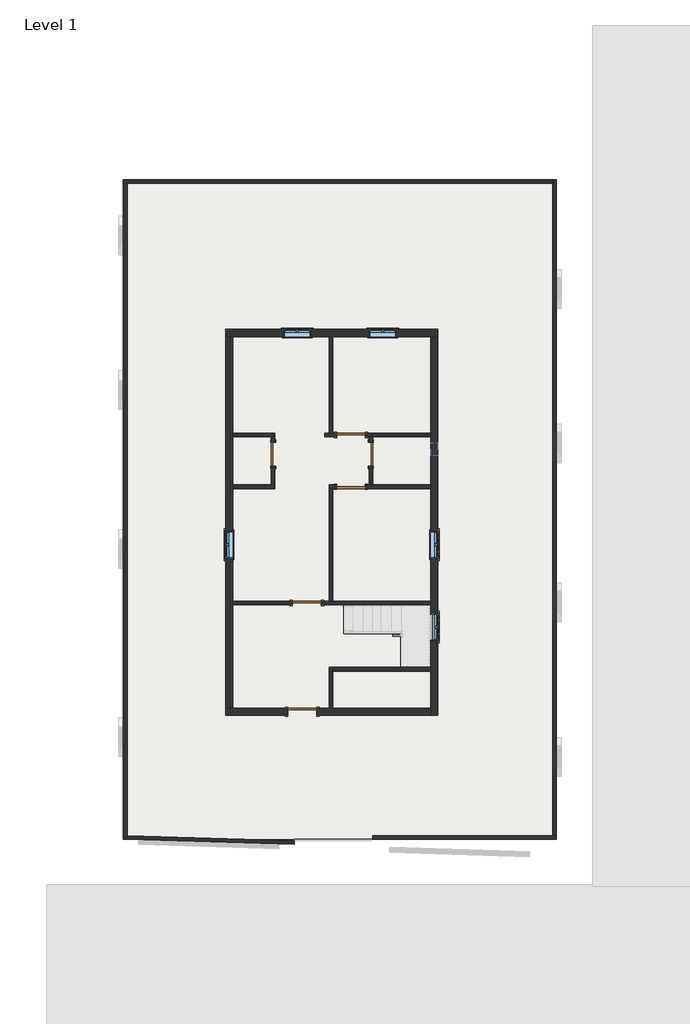
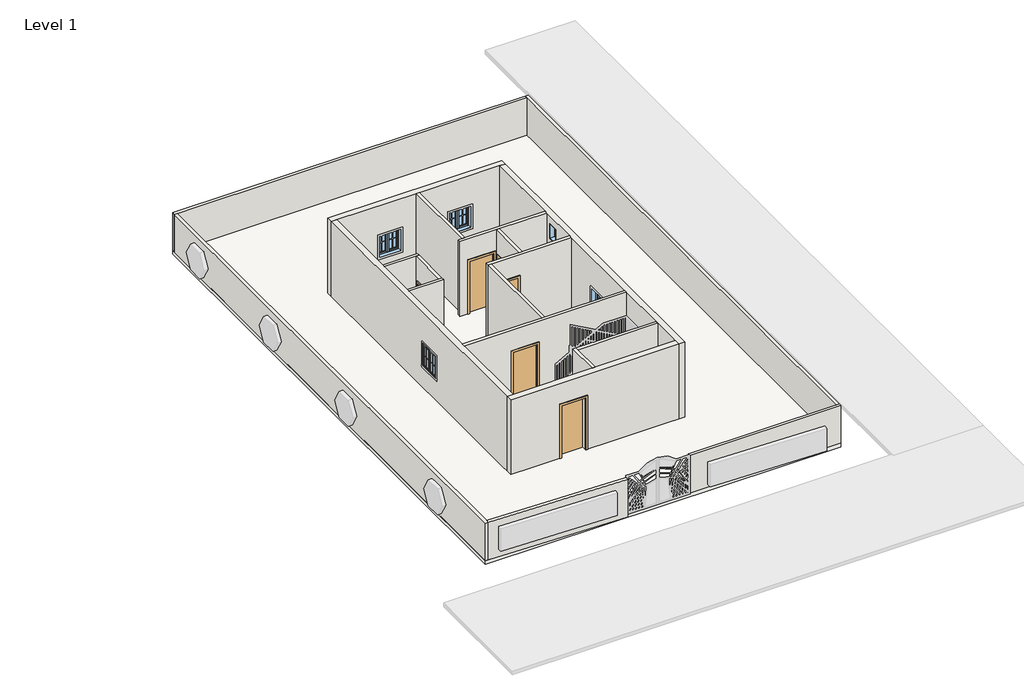
# One storey, part 1 of 3: 20 walls, 6 doors, 6 windows, 1 slab.
"""IFC4 building model written with IfcOpenShell, lengths in millimetres."""

from ifc_helpers import new_model, si_unit, frame, origin, origin_with_axes, place, context, project, spatial, polyline, outline, extrude, faceted_brep, transform, mapped, element, save
from components import door_f2b275c1, door_d8f5dbb5, door_305aa2a5, door_e5f9f3c4, door_a90ba1ad, window_aa618e30, window_339605e1

model = new_model("IFC4")

# Units and contexts
model_context = context("Model", 3, world=origin())
ifc_project = project(units=[si_unit("LENGTHUNIT", "METRE", prefix="MILLI")], contexts=[model_context])

# Site, building, storey
site = spatial("IfcSite", under=ifc_project)
building = spatial("IfcBuilding", under=site)
storey = spatial("IfcBuildingStorey", under=building, Name="Level 1", Elevation=0.0)

# Doors
placement = place(None, origin())
door_shape = door_f2b275c1(model_context)
element("IfcDoor", 1, ObjectType="Single-Flush : 30\" x 80\"", at=placement, inside=storey, context=model_context, shape_type="MappedRepresentation", body=[
    mapped(door_shape, transform((-22.290747, 2690.8435985, 0.0), x_axis=(0.0, 1.0, 0.0), y_axis=(-1.0, 0.0, 0.0), z_axis=(0.0, 0.0, 1.0))),
])
door_2_shape = door_d8f5dbb5(model_context)
element("IfcDoor", 2, ObjectType="Single-Flush : 30\" x 80\"", at=placement, inside=storey, context=model_context, shape_type="MappedRepresentation", body=[
    mapped(door_2_shape, transform((-3108.390747, 2690.8435985, 0.0), x_axis=(0.0, 1.0, 0.0), y_axis=(-1.0, 0.0, 0.0), z_axis=(0.0, 0.0, 1.0))),
])
door_3_shape = door_305aa2a5(model_context)
element("IfcDoor", 3, ObjectType="Single-Flush : 36\" x 84\"", at=placement, inside=storey, context=model_context, shape_type="MappedRepresentation", body=[
    mapped(door_3_shape, transform((-650.940747, 3300.4435985, 0.0), x_axis=(-1.0, 0.0, 0.0), y_axis=(0.0, -1.0, 0.0), z_axis=(0.0, 0.0, 1.0))),
])
door_4_shape = door_e5f9f3c4(model_context)
element("IfcDoor", 4, ObjectType="Single-Flush : 36\" x 84\"", at=placement, inside=storey, context=model_context, shape_type="MappedRepresentation", body=[
    mapped(door_4_shape, transform((-2041.590747, -2008.1564015, 0.0), x_axis=(1.0, 0.0, 0.0), y_axis=(0.0, 1.0, 0.0), z_axis=(0.0, 0.0, 1.0))),
])
element("IfcDoor", 5, ObjectType="Single-Flush : 36\" x 84\"", at=placement, inside=storey, context=model_context, shape_type="MappedRepresentation", body=[
    mapped(door_4_shape, transform((-650.940747, 1662.1435985, 0.0), x_axis=(-1.0, 0.0, 0.0), y_axis=(0.0, -1.0, 0.0), z_axis=(0.0, 0.0, 1.0))),
])
door_5_shape = door_a90ba1ad(model_context)
element("IfcDoor", 6, ObjectType="Single-Flush : 36\" x 84\"", at=placement, inside=storey, context=model_context, shape_type="MappedRepresentation", body=[
    mapped(door_5_shape, transform((-2193.990747, -5443.5064015, 0.0), x_axis=(-1.0, 0.0, 0.0), y_axis=(0.0, -1.0, 0.0), z_axis=(0.0, 0.0, 1.0))),
])

# Slab
element("IfcSlab", 7, ObjectType="Generic - 12\"", at=placement, inside=storey, context=model_context, shape_type="SweptSolid", body=[
    extrude(outline(polyline([(5837.7486397, 11368.6225468), (5837.7486397, -9472.0774532), (-7840.1513603, -9472.0774532), (-7840.1513603, 11368.6225468), (5837.7486397, 11368.6225468)])), frame((0.0, 0.0, -152.4), z_axis=(0.0, 0.0, 1.0), x_axis=(1.0, 0.0, 0.0)), (0.0, 0.0, 1.0), 152.4),
])

# Walls
element("IfcWall", 8, ObjectType="WALL4.5\"", at=placement, inside=storey, context=model_context, shape_type="Brep", body=[
    faceted_brep([(-4384.740747, 3243.2935985, 0.0), (-3165.540747, 3243.2935985, 0.0), (-3051.240747, 3243.2935985, 0.0), (-3051.240747, 3243.2935985, 3048.0), (-3165.540747, 3243.2935985, 3048.0), (-4384.740747, 3243.2935985, 3048.0), (-4384.740747, 3357.5935985, 0.0), (-4384.740747, 3357.5935985, 3048.0), (-3051.240747, 3357.5935985, 3048.0), (-3051.240747, 3357.5935985, 0.0)], [[[0, 1, 2, 3, 4, 5]], [[6, 7, 8, 9]], [[2, 1, 0, 6, 9]], [[0, 5, 7, 6]], [[3, 2, 9, 8]], [[5, 4, 3, 8, 7]]]),
])
element("IfcWall", 9, ObjectType="WALL4.5\"", at=placement, inside=storey, context=model_context, shape_type="Brep", body=[
    faceted_brep([(-4384.740747, 1604.9935985, 0.0), (-3051.240747, 1604.9935985, 0.0), (-3051.240747, 1604.9935985, 3048.0), (-4384.740747, 1604.9935985, 3048.0), (-4384.740747, 1719.2935985, 0.0), (-4384.740747, 1719.2935985, 3048.0), (-3165.540747, 1719.2935985, 3048.0), (-3051.240747, 1719.2935985, 3048.0), (-3051.240747, 1719.2935985, 0.0), (-3165.540747, 1719.2935985, 0.0)], [[[0, 1, 2, 3]], [[4, 5, 6, 7, 8, 9]], [[1, 0, 4, 9, 8]], [[0, 3, 5, 4]], [[2, 1, 8, 7]], [[3, 2, 7, 6, 5]]]),
])
element("IfcWall", 10, ObjectType="WALL4.5\"", at=placement, inside=storey, context=model_context, shape_type="SweptSolid", body=[
    extrude(outline(polyline([(3243.2935985, 0.0), (3071.8435985, 0.0), (3071.8435985, 2032.0), (2309.8435985, 2032.0), (2309.8435985, 0.0), (1719.2935985, 0.0), (1719.2935985, 3048.0), (3243.2935985, 3048.0), (3243.2935985, 0.0)])), frame((-3165.540747, 0.0, 0.0), z_axis=(1.0, 0.0, 0.0), x_axis=(0.0, 1.0, 0.0)), (0.0, 0.0, 1.0), 114.3),
])
element("IfcWall", 11, ObjectType="WALL4.5\"", at=placement, inside=storey, context=model_context, shape_type="SweptSolid", body=[
    extrude(outline(polyline([(-1336.740747, 3357.5935985), (-1336.740747, 6405.5935985), (-1222.440747, 6405.5935985), (-1222.440747, 3357.5935985), (-1336.740747, 3357.5935985)])), origin_with_axes(), (0.0, 0.0, 1.0), 3048.0),
])
element("IfcWall", 12, ObjectType="WALL4.5\"", at=placement, inside=storey, context=model_context, shape_type="Brep", body=[
    faceted_brep([(-1481.7019184, 3243.2935985, 0.0), (-1108.140747, 3243.2935985, 0.0), (-1108.140747, 3243.2935985, 2133.6), (-193.740747, 3243.2935985, 2133.6), (-193.740747, 3243.2935985, 0.0), (-79.440747, 3243.2935985, 0.0), (34.859253, 3243.2935985, 0.0), (1863.659253, 3243.2935985, 0.0), (1863.659253, 3243.2935985, 3048.0), (34.859253, 3243.2935985, 3048.0), (-79.440747, 3243.2935985, 3048.0), (-1481.7019184, 3243.2935985, 3048.0), (-1108.140747, 3357.5935985, 2133.6), (-1108.140747, 3357.5935985, 0.0), (-1222.440747, 3357.5935985, 0.0), (-1336.740747, 3357.5935985, 0.0), (-1481.7019184, 3357.5935985, 0.0), (-1481.7019184, 3357.5935985, 3048.0), (-1336.740747, 3357.5935985, 3048.0), (-1222.440747, 3357.5935985, 3048.0), (1863.659253, 3357.5935985, 3048.0), (1863.659253, 3357.5935985, 0.0), (-193.740747, 3357.5935985, 0.0), (-193.740747, 3357.5935985, 2133.6)], [[[0, 1, 2, 3, 4, 5, 6, 7, 8, 9, 10, 11]], [[12, 13, 14, 15, 16, 17, 18, 19, 20, 21, 22, 23]], [[22, 21, 7, 6, 5, 4]], [[16, 15, 14, 13, 1, 0]], [[0, 11, 17, 16]], [[8, 7, 21, 20]], [[2, 1, 13, 12]], [[3, 2, 12, 23]], [[4, 3, 23, 22]], [[11, 10, 9, 8, 20, 19, 18, 17]]]),
])
element("IfcWall", 13, ObjectType="WALL4.5\"", at=placement, inside=storey, context=model_context, shape_type="SweptSolid", body=[
    extrude(outline(polyline([(3243.2935985, 0.0), (3071.8435985, 0.0), (3071.8435985, 2032.0), (2309.8435985, 2032.0), (2309.8435985, 0.0), (1719.2935985, 0.0), (1719.2935985, 3048.0), (3243.2935985, 3048.0), (3243.2935985, 0.0)])), frame((-79.440747, 0.0, 0.0), z_axis=(1.0, 0.0, 0.0), x_axis=(0.0, 1.0, 0.0)), (0.0, 0.0, 1.0), 114.3),
])
element("IfcWall", 14, ObjectType="WALL4.5\"", at=placement, inside=storey, context=model_context, shape_type="Brep", body=[
    faceted_brep([(-1108.140747, 1719.2935985, 2133.6), (-1108.140747, 1719.2935985, 0.0), (-1336.740747, 1719.2935985, 0.0), (-1336.740747, 1719.2935985, 3048.0), (-79.440747, 1719.2935985, 3048.0), (34.859253, 1719.2935985, 3048.0), (1863.659253, 1719.2935985, 3048.0), (1863.659253, 1719.2935985, 0.0), (34.859253, 1719.2935985, 0.0), (-79.440747, 1719.2935985, 0.0), (-193.740747, 1719.2935985, 0.0), (-193.740747, 1719.2935985, 2133.6), (-1336.740747, 1604.9935985, 0.0), (-1222.440747, 1604.9935985, 0.0), (-1108.140747, 1604.9935985, 0.0), (-1108.140747, 1604.9935985, 2133.6), (-193.740747, 1604.9935985, 2133.6), (-193.740747, 1604.9935985, 0.0), (1863.659253, 1604.9935985, 0.0), (1863.659253, 1604.9935985, 3048.0), (-1222.440747, 1604.9935985, 3048.0), (-1336.740747, 1604.9935985, 3048.0)], [[[0, 1, 2, 3, 4, 5, 6, 7, 8, 9, 10, 11]], [[12, 13, 14, 15, 16, 17, 18, 19, 20, 21]], [[2, 1, 14, 13, 12]], [[10, 9, 8, 7, 18, 17]], [[7, 6, 19, 18]], [[3, 2, 12, 21]], [[15, 14, 1, 0]], [[16, 15, 0, 11]], [[17, 16, 11, 10]], [[6, 5, 4, 3, 21, 20, 19]]]),
])
element("IfcWall", 15, ObjectType="WALL4.5\"", at=placement, inside=storey, context=model_context, shape_type="SweptSolid", body=[
    extrude(outline(polyline([(-1336.740747, -1951.0064015), (-1336.740747, 1604.9935985), (-1222.440747, 1604.9935985), (-1222.440747, -1951.0064015), (-1336.740747, -1951.0064015)])), origin_with_axes(), (0.0, 0.0, 1.0), 3048.0),
])
element("IfcWall", 16, ObjectType="WALL4.5\"", at=placement, inside=storey, context=model_context, shape_type="Brep", body=[
    faceted_brep([(-1584.390747, -2065.3064015, 2133.6), (-1584.390747, -2065.3064015, 0.0), (1863.659253, -2065.3064015, 0.0), (1863.659253, -2065.3064015, 3048.0), (-4384.740747, -2065.3064015, 3048.0), (-4384.740747, -2065.3064015, 0.0), (-2498.790747, -2065.3064015, 0.0), (-2498.790747, -2065.3064015, 2133.6), (1863.659253, -1951.0064015, 0.0), (-1222.440747, -1951.0064015, 0.0), (-1336.740747, -1951.0064015, 0.0), (-1584.390747, -1951.0064015, 0.0), (-1584.390747, -1951.0064015, 2133.6), (-2498.790747, -1951.0064015, 2133.6), (-2498.790747, -1951.0064015, 0.0), (-4384.740747, -1951.0064015, 0.0), (-4384.740747, -1951.0064015, 3048.0), (-1336.740747, -1951.0064015, 3048.0), (-1222.440747, -1951.0064015, 3048.0), (1863.659253, -1951.0064015, 3048.0)], [[[0, 1, 2, 3, 4, 5, 6, 7]], [[8, 9, 10, 11, 12, 13, 14, 15, 16, 17, 18, 19]], [[6, 5, 15, 14]], [[2, 1, 11, 10, 9, 8]], [[3, 2, 8, 19]], [[5, 4, 16, 15]], [[12, 11, 1, 0]], [[13, 12, 0, 7]], [[14, 13, 7, 6]], [[4, 3, 19, 18, 17, 16]]]),
])
element("IfcWall", 17, ObjectType="WALL4.5\"", at=placement, inside=storey, context=model_context, shape_type="Brep", body=[
    faceted_brep([(-1222.440747, -5329.2064015, 0.0), (-1222.440747, -4160.8064015, 0.0), (-1222.440747, -4046.5064015, 0.0), (-1222.440747, -4046.5064015, 3048.0), (-1222.440747, -4160.8064015, 3048.0), (-1222.440747, -5329.2064015, 3048.0), (-1336.740747, -5329.2064015, 0.0), (-1336.740747, -5329.2064015, 3048.0), (-1336.740747, -4046.5064015, 3048.0), (-1336.740747, -4046.5064015, 0.0)], [[[0, 1, 2, 3, 4, 5]], [[6, 7, 8, 9]], [[2, 1, 0, 6, 9]], [[0, 5, 7, 6]], [[3, 2, 9, 8]], [[5, 4, 3, 8, 7]]]),
])
element("IfcWall", 18, ObjectType="WALL4.5\"", at=placement, inside=storey, context=model_context, shape_type="SweptSolid", body=[
    extrude(outline(polyline([(1863.659253, -4160.8064015), (-1222.440747, -4160.8064015), (-1222.440747, -4046.5064015), (1863.659253, -4046.5064015), (1863.659253, -4160.8064015)])), origin_with_axes(), (0.0, 0.0, 1.0), 3048.0),
])
element("IfcWall", 19, ObjectType="WALL4.5\"", at=placement, inside=storey, context=model_context, shape_type="Brep", body=[
    faceted_brep([(-7840.1513603, 11254.3225468, 0.0), (-7725.8513603, 11254.3225468, 0.0), (5723.4486397, 11254.3225468, 0.0), (5723.4486397, 11254.3225468, 1524.0), (-7725.8513603, 11254.3225468, 1524.0), (-7840.1513603, 11254.3225468, 1524.0), (-7840.1513603, 11368.6225468, 0.0), (-7840.1513603, 11368.6225468, 1524.0), (5723.4486397, 11368.6225468, 1524.0), (5723.4486397, 11368.6225468, 0.0)], [[[0, 1, 2, 3, 4, 5]], [[6, 7, 8, 9]], [[2, 1, 0, 6, 9]], [[5, 4, 3, 8, 7]], [[0, 5, 7, 6]], [[3, 2, 9, 8]]]),
])
element("IfcWall", 20, ObjectType="WALL4.5\"", at=placement, inside=storey, context=model_context, shape_type="Brep", body=[
    faceted_brep([(-7725.8513603, -9473.8996485, 0.0), (-7725.8513603, -9359.5449948, 0.0), (-7725.8513603, 11254.3225468, 0.0), (-7725.8513603, 11254.3225468, 1524.0), (-7725.8513603, -9359.5449948, 1524.0), (-7725.8513603, -9473.8996485, 1524.0), (-7840.1513603, -9470.3645653, 0.0), (-7840.1513603, -9470.3645653, 1524.0), (-7840.1513603, 11254.3225468, 1524.0), (-7840.1513603, 11254.3225468, 0.0)], [[[0, 1, 2, 3, 4, 5]], [[6, 7, 8, 9]], [[2, 1, 0, 6, 9]], [[5, 4, 3, 8, 7]], [[0, 5, 7, 6]], [[3, 2, 9, 8]]]),
])
element("IfcWall", 21, ObjectType="WALL4.5\"", at=placement, inside=storey, context=model_context, shape_type="Brep", body=[
    faceted_brep([(5837.7486397, -9357.7774532, 0.0), (5723.4486397, -9357.7774532, 0.0), (40.1986397, -9357.7774532, 0.0), (40.1986397, -9357.7774532, 1524.0), (5723.4486397, -9357.7774532, 1524.0), (5837.7486397, -9357.7774532, 1524.0), (5837.7486397, -9472.0774532, 0.0), (5837.7486397, -9472.0774532, 1524.0), (40.1986397, -9472.0774532, 1524.0), (40.1986397, -9472.0774532, 0.0)], [[[0, 1, 2, 3, 4, 5]], [[6, 7, 8, 9]], [[2, 1, 0, 6, 9]], [[3, 2, 9, 8]], [[5, 4, 3, 8, 7]], [[0, 5, 7, 6]]]),
])
element("IfcWall", 22, ObjectType="WALL4.5\"", at=placement, inside=storey, context=model_context, shape_type="Brep", body=[
    faceted_brep([(5723.4486397, 11368.6225468, 0.0), (5723.4486397, 11254.3225468, 0.0), (5723.4486397, -9357.7774532, 0.0), (5723.4486397, -9357.7774532, 1524.0), (5723.4486397, 11254.3225468, 1524.0), (5723.4486397, 11368.6225468, 1524.0), (5837.7486397, 11368.6225468, 0.0), (5837.7486397, 11368.6225468, 1524.0), (5837.7486397, -9357.7774532, 1524.0), (5837.7486397, -9357.7774532, 0.0)], [[[0, 1, 2, 3, 4, 5]], [[6, 7, 8, 9]], [[2, 1, 0, 6, 9]], [[5, 4, 3, 8, 7]], [[0, 5, 7, 6]], [[3, 2, 9, 8]]]),
])
element("IfcWall", 23, ObjectType="WALL4.5\"", at=placement, inside=storey, context=model_context, shape_type="SweptSolid", body=[
    extrude(outline(polyline([(-7725.8513603, -9359.5449948), (-2444.815747, -9522.8774532), (-2448.3491406, -9637.1228257), (-7725.8513603, -9473.8996485), (-7725.8513603, -9359.5449948)])), origin_with_axes(), (0.0, 0.0, 1.0), 1524.0),
])
element("IfcWall", 24, ObjectType="WALL9\"", at=placement, inside=storey, context=model_context, shape_type="Brep", body=[
    faceted_brep([(-4613.340747, 6405.5935985, 0.0), (-4384.740747, 6405.5935985, 0.0), (-1336.740747, 6405.5935985, 0.0), (-1222.440747, 6405.5935985, 0.0), (1863.659253, 6405.5935985, 0.0), (2092.259253, 6405.5935985, 0.0), (2092.259253, 6405.5935985, 3048.0), (1863.659253, 6405.5935985, 3048.0), (-1222.440747, 6405.5935985, 3048.0), (-1336.740747, 6405.5935985, 3048.0), (-4384.740747, 6405.5935985, 3048.0), (-4613.340747, 6405.5935985, 3048.0), (-1914.590747, 6405.5935985, 1828.8), (-1914.590747, 6405.5935985, 914.4), (-2778.190747, 6405.5935985, 914.4), (-2778.190747, 6405.5935985, 1828.8), (780.984253, 6405.5935985, 1828.8), (780.984253, 6405.5935985, 914.4), (-82.615747, 6405.5935985, 914.4), (-82.615747, 6405.5935985, 1828.8), (-4613.340747, 6634.1935985, 0.0), (-4613.340747, 6634.1935985, 3048.0), (2092.259253, 6634.1935985, 3048.0), (2092.259253, 6634.1935985, 0.0), (-1914.590747, 6634.1935985, 1828.8), (-2778.190747, 6634.1935985, 1828.8), (-2778.190747, 6634.1935985, 914.4), (-1914.590747, 6634.1935985, 914.4), (780.984253, 6634.1935985, 1828.8), (-82.615747, 6634.1935985, 1828.8), (-82.615747, 6634.1935985, 914.4), (780.984253, 6634.1935985, 914.4)], [[[0, 1, 2, 3, 4, 5, 6, 7, 8, 9, 10, 11], [12, 13, 14, 15], [16, 17, 18, 19]], [[20, 21, 22, 23], [24, 25, 26, 27], [28, 29, 30, 31]], [[5, 4, 3, 2, 1, 0, 20, 23]], [[6, 5, 23, 22]], [[0, 11, 21, 20]], [[13, 12, 24, 27]], [[14, 13, 27, 26]], [[15, 14, 26, 25]], [[12, 15, 25, 24]], [[17, 16, 28, 31]], [[18, 17, 31, 30]], [[19, 18, 30, 29]], [[16, 19, 29, 28]], [[11, 10, 9, 8, 7, 6, 22, 21]]]),
])
element("IfcWall", 25, ObjectType="WALL9\"", at=placement, inside=storey, context=model_context, shape_type="Brep", body=[
    faceted_brep([(1863.659253, 6405.5935985, 0.0), (1863.659253, 3357.5935985, 0.0), (1863.659253, 3243.2935985, 0.0), (1863.659253, 1719.2935985, 0.0), (1863.659253, 1604.9935985, 0.0), (1863.659253, -1951.0064015, 0.0), (1863.659253, -2065.3064015, 0.0), (1863.659253, -4046.5064015, 0.0), (1863.659253, -4160.8064015, 0.0), (1863.659253, -5329.2064015, 0.0), (1863.659253, -5557.8064015, 0.0), (1863.659253, -5557.8064015, 3048.0), (1863.659253, -5329.2064015, 3048.0), (1863.659253, -4160.8064015, 3048.0), (1863.659253, -4046.5064015, 3048.0), (1863.659253, -2065.3064015, 3048.0), (1863.659253, -1951.0064015, 3048.0), (1863.659253, 1604.9935985, 3048.0), (1863.659253, 1719.2935985, 3048.0), (1863.659253, 3243.2935985, 3048.0), (1863.659253, 3357.5935985, 3048.0), (1863.659253, 6405.5935985, 3048.0), (1863.659253, 2640.0435985, 2743.2), (1863.659253, 2640.0435985, 2133.6), (1863.659253, 3046.4435985, 2133.6), (1863.659253, 3046.4435985, 2743.2), (1863.659253, -604.8064015, 1828.8), (1863.659253, -604.8064015, 914.4), (1863.659253, 258.7935985, 914.4), (1863.659253, 258.7935985, 1828.8), (1863.659253, -3201.9564015, 1828.8), (1863.659253, -3201.9564015, 914.4), (1863.659253, -2338.3564015, 914.4), (1863.659253, -2338.3564015, 1828.8), (2092.259253, 6405.5935985, 0.0), (2092.259253, 6405.5935985, 3048.0), (2092.259253, -5557.8064015, 3048.0), (2092.259253, -5557.8064015, 0.0), (2092.259253, 2640.0435985, 2743.2), (2092.259253, 3046.4435985, 2743.2), (2092.259253, 3046.4435985, 2133.6), (2092.259253, 2640.0435985, 2133.6), (2092.259253, -604.8064015, 1828.8), (2092.259253, 258.7935985, 1828.8), (2092.259253, 258.7935985, 914.4), (2092.259253, -604.8064015, 914.4), (2092.259253, -3201.9564015, 1828.8), (2092.259253, -2338.3564015, 1828.8), (2092.259253, -2338.3564015, 914.4), (2092.259253, -3201.9564015, 914.4)], [[[0, 1, 2, 3, 4, 5, 6, 7, 8, 9, 10, 11, 12, 13, 14, 15, 16, 17, 18, 19, 20, 21], [22, 23, 24, 25], [26, 27, 28, 29], [30, 31, 32, 33]], [[34, 35, 36, 37], [38, 39, 40, 41], [42, 43, 44, 45], [46, 47, 48, 49]], [[10, 9, 8, 7, 6, 5, 4, 3, 2, 1, 0, 34, 37]], [[0, 21, 35, 34]], [[11, 10, 37, 36]], [[23, 22, 38, 41]], [[24, 23, 41, 40]], [[25, 24, 40, 39]], [[22, 25, 39, 38]], [[27, 26, 42, 45]], [[28, 27, 45, 44]], [[29, 28, 44, 43]], [[26, 29, 43, 42]], [[31, 30, 46, 49]], [[32, 31, 49, 48]], [[33, 32, 48, 47]], [[30, 33, 47, 46]], [[21, 20, 19, 18, 17, 16, 15, 14, 13, 12, 11, 36, 35]]]),
])
element("IfcWall", 26, ObjectType="WALL9\"", at=placement, inside=storey, context=model_context, shape_type="Brep", body=[
    faceted_brep([(-2651.190747, -5329.2064015, 2133.6), (-2651.190747, -5329.2064015, 0.0), (-4384.740747, -5329.2064015, 0.0), (-4613.340747, -5329.2064015, 0.0), (-4613.340747, -5329.2064015, 3048.0), (-4384.740747, -5329.2064015, 3048.0), (-1336.740747, -5329.2064015, 3048.0), (-1222.440747, -5329.2064015, 3048.0), (1863.659253, -5329.2064015, 3048.0), (1863.659253, -5329.2064015, 0.0), (-1222.440747, -5329.2064015, 0.0), (-1336.740747, -5329.2064015, 0.0), (-1736.790747, -5329.2064015, 0.0), (-1736.790747, -5329.2064015, 2133.6), (-4613.340747, -5557.8064015, 0.0), (-2651.190747, -5557.8064015, 0.0), (-2651.190747, -5557.8064015, 2133.6), (-1736.790747, -5557.8064015, 2133.6), (-1736.790747, -5557.8064015, 0.0), (1863.659253, -5557.8064015, 0.0), (1863.659253, -5557.8064015, 3048.0), (-4613.340747, -5557.8064015, 3048.0)], [[[0, 1, 2, 3, 4, 5, 6, 7, 8, 9, 10, 11, 12, 13]], [[14, 15, 16, 17, 18, 19, 20, 21]], [[3, 2, 1, 15, 14]], [[12, 11, 10, 9, 19, 18]], [[9, 8, 20, 19]], [[4, 3, 14, 21]], [[16, 15, 1, 0]], [[17, 16, 0, 13]], [[18, 17, 13, 12]], [[8, 7, 6, 5, 4, 21, 20]]]),
])
element("IfcWall", 27, ObjectType="WALL9\"", at=placement, inside=storey, context=model_context, shape_type="Brep", body=[
    faceted_brep([(-4384.740747, -5329.2064015, 0.0), (-4384.740747, -2065.3064015, 0.0), (-4384.740747, -1951.0064015, 0.0), (-4384.740747, 1604.9935985, 0.0), (-4384.740747, 1719.2935985, 0.0), (-4384.740747, 3243.2935985, 0.0), (-4384.740747, 3357.5935985, 0.0), (-4384.740747, 6405.5935985, 0.0), (-4384.740747, 6405.5935985, 3048.0), (-4384.740747, 3357.5935985, 3048.0), (-4384.740747, 3243.2935985, 3048.0), (-4384.740747, 1719.2935985, 3048.0), (-4384.740747, 1604.9935985, 3048.0), (-4384.740747, -1951.0064015, 3048.0), (-4384.740747, -2065.3064015, 3048.0), (-4384.740747, -5329.2064015, 3048.0), (-4384.740747, 258.7935985, 1828.8), (-4384.740747, 258.7935985, 914.4), (-4384.740747, -604.8064015, 914.4), (-4384.740747, -604.8064015, 1828.8), (-4613.340747, -5329.2064015, 0.0), (-4613.340747, -5329.2064015, 3048.0), (-4613.340747, 6405.5935985, 3048.0), (-4613.340747, 6405.5935985, 0.0), (-4613.340747, 258.7935985, 1828.8), (-4613.340747, -604.8064015, 1828.8), (-4613.340747, -604.8064015, 914.4), (-4613.340747, 258.7935985, 914.4)], [[[0, 1, 2, 3, 4, 5, 6, 7, 8, 9, 10, 11, 12, 13, 14, 15], [16, 17, 18, 19]], [[20, 21, 22, 23], [24, 25, 26, 27]], [[7, 6, 5, 4, 3, 2, 1, 0, 20, 23]], [[8, 7, 23, 22]], [[0, 15, 21, 20]], [[17, 16, 24, 27]], [[18, 17, 27, 26]], [[19, 18, 26, 25]], [[16, 19, 25, 24]], [[15, 14, 13, 12, 11, 10, 9, 8, 22, 21]]]),
])

# Windows
window_shape = window_aa618e30(model_context)
element("IfcWindow", 28, ObjectType="Fixed : 16\" x 24\"", at=placement, inside=storey, context=model_context, shape_type="MappedRepresentation", body=[
    mapped(window_shape, transform((1977.959253, 2805.1435985, 1219.2), x_axis=(0.0, -1.0, 0.0), y_axis=(1.0, 0.0, 0.0), z_axis=(0.0, 0.0, 1.0))),
])
window_2_shape = window_339605e1(model_context)
element("IfcWindow", 29, ObjectType="Window-Casement-Double : 34\" x 36\"", at=placement, inside=storey, context=model_context, shape_type="MappedRepresentation", body=[
    mapped(window_2_shape, transform((-2346.390747, 6519.8935985, 0.0), x_axis=(1.0, 0.0, 0.0), y_axis=(0.0, 1.0, 0.0), z_axis=(0.0, 0.0, 1.0))),
])
element("IfcWindow", 30, ObjectType="Window-Casement-Double : 34\" x 36\"", at=placement, inside=storey, context=model_context, shape_type="MappedRepresentation", body=[
    mapped(window_2_shape, transform((349.184253, 6519.8935985, 0.0), x_axis=(1.0, 0.0, 0.0), y_axis=(0.0, 1.0, 0.0), z_axis=(0.0, 0.0, 1.0))),
])
element("IfcWindow", 31, ObjectType="Window-Casement-Double : 34\" x 36\"", at=placement, inside=storey, context=model_context, shape_type="MappedRepresentation", body=[
    mapped(window_2_shape, transform((1977.959253, -173.0064015, 0.0), x_axis=(0.0, -1.0, 0.0), y_axis=(1.0, 0.0, 0.0), z_axis=(0.0, 0.0, 1.0))),
])
element("IfcWindow", 32, ObjectType="Window-Casement-Double : 34\" x 36\"", at=placement, inside=storey, context=model_context, shape_type="MappedRepresentation", body=[
    mapped(window_2_shape, transform((-4499.040747, -173.0064015, 0.0), x_axis=(0.0, 1.0, 0.0), y_axis=(-1.0, 0.0, 0.0), z_axis=(0.0, 0.0, 1.0))),
])
element("IfcWindow", 33, ObjectType="Window-Casement-Double : 34\" x 36\"", at=placement, inside=storey, context=model_context, shape_type="MappedRepresentation", body=[
    mapped(window_2_shape, transform((1977.959253, -2770.1564015, 0.0), x_axis=(0.0, -1.0, 0.0), y_axis=(1.0, 0.0, 0.0), z_axis=(0.0, 0.0, 1.0))),
])

save(model, "model.ifc")

# Revit data of these elements
# Type "Single-Flush : 30\" x 80\""
#   Type Mark = "5"
#   Construction Type Id = "MDOOR"
#   Assembly Code = "C1020"
#   Analytic Construction = "Metal"
#   Thickness = 0' - 2"
#   Heat Transfer Coefficient (U) = 0.651978 BTU/(h·ft²·°F)
#   Height = 6' - 8"
#   Trim Projection Ext = 0' - 1"
#   Trim Projection Int = 0' - 1"
#   Trim Width = 0' - 3"
#   Width = 2' - 6"
#   Define Thermal Properties by = 1
#   Define Thermal Properties by = 1
#   Door Material = Door - Panel
#   Frame Material = Door - Frame
#   Visual Light Transmittance = 0
#   Solar Heat Gain Coefficient = 0
#   Function = (empty or 0)
#   Wall Closure = (empty or 0)
# Type "Single-Flush : 36\" x 84\""
#   Type Mark = "1"
#   Construction Type Id = "MDOOR"
#   Assembly Code = "C1020"
#   Analytic Construction = "Metal"
#   Thickness = 0' - 2"
#   Heat Transfer Coefficient (U) = 0.651978 BTU/(h·ft²·°F)
#   Height = 7' - 0"
#   Trim Projection Ext = 0' - 1"
#   Trim Projection Int = 0' - 1"
#   Trim Width = 0' - 3"
#   Width = 3' - 0"
#   Define Thermal Properties by = 1
#   Define Thermal Properties by = 1
#   Door Material = Door - Panel
#   Frame Material = Door - Frame
#   Visual Light Transmittance = 0
#   Solar Heat Gain Coefficient = 0
#   Function = (empty or 0)
#   Wall Closure = (empty or 0)
# Type "Generic - 12\""
#   Assembly Code = "B1010"
#   Function = 0
#   Layers, outside or top first: 0' - 6" no material (function 1)
# Type "WALL4.5\""
#   Assembly Code = "B2010"
#   Layers, outside or top first: 0' - 4 1/2" no material (function 1)
# Type "WALL9\""
#   Assembly Code = "B2010"
#   Layers, outside or top first: 0' - 9" no material (function 1)
# Type "Fixed : 16\" x 24\""
#   Type Mark = "4"
#   Construction Type Id = "GSP4R"
#   Assembly Code = "B2020100"
#   Analytic Construction = "1/8 in Pilkington single glazing"
#   Visual Light Transmittance = 0.9
#   Solar Heat Gain Coefficient = 0.78
#   Heat Transfer Coefficient (U) = 0.6496 BTU/(h·ft²·°F)
#   Height = 2' - 0"
#   Default Sill Height = 3' - 0"
#   Width = 1' - 4"
#   Window Inset = 0' - 0 3/4"
#   Define Thermal Properties by = 1
#   Define Thermal Properties by = 1
#   Glass Pane Material = Glass
#   Sash Material = Sash
#   Wall Closure = (empty or 0)
# Type "Window-Casement-Double : 34\" x 36\""
#   Type Mark = "14"
#   Fire Rating = "0.5h"
#   Assembly Code = "B2020100"
#   Analytic Construction = "Double glazing - domestic"
#   Frame Extension [instance default] = 0' - 0 1/4"
#   Window Inset [instance default] = 0' - 0"
#   Wall Thickness [instance default] = 0' - 6"
#   Interior Wall Closure [instance default] = 0' - 2 1/4"
#   Half Width = 1' - 5"
#   Visual Light Transmittance = 0.81
#   Thermal Resistance (R) = 1.8146 (h·ft²·°F)/BTU
#   Solar Heat Gain Coefficient = 0.76
#   Rough Width = 2' - 10 1/2"
#   Rough Height = 3' - 0 1/2"
#   Height = 3' - 0"
#   Heat Transfer Coefficient (U) = 0.5511 BTU/(h·ft²·°F)
#   Exterior Wall Closure [instance default] = 0' - 1 1/4"
#   Extension Jamb [instance default] = 0' - 2 1/4"
#   Default Sill Height = 3' - 0"
#   Width = 2' - 10"
#   Define Thermal Properties by = 0
#   Muntin Visibility = yes
#   Interior Trim Visibility [instance default] = yes
#   Exterior Trim Visibility [instance default] = yes
#   Extension Jamb Visibility [instance default] = yes
#   Interior Trim Material = Wood - Stained
#   Muntin Pattern = Muntin Pattern_2x2 : Muntin Pattern_2x2
#   Interior Trim = Trim-Window-Interior-Flat : Picture Frame
#   Interior Frame Material = Wood - Stained
#   Glass Panel Material = Glass
#   Exterior Trim Material = Clad - White
#   Exterior Trim = Trim-Window-Exterior-Flat : with Sill
#   Exterior Frame Material = Clad - White
#   Wall Closure = (empty or 0)
# Elements 1, 2 (IfcDoor, "Single-Flush : 30\" x 80\"")
#   Phase Created = New Construction
#   Materials on its faces: "Door - Frame", "Door - Panel"
# Elements 3, 4, 5, 6 (IfcDoor, "Single-Flush : 36\" x 84\"")
#   Phase Created = New Construction
#   Materials on its faces: "Door - Frame", "Door - Panel"
# Element 7 (IfcSlab, "Generic - 12\"")
#   Height Offset From Level = 0' - 0"
#   Phase Created = New Construction
#   Materials on its faces: "Default Floor"
# Elements 8, 9, 10, 11, 12, 13, 14, 15, 16, 17, 18 (IfcWall, "WALL4.5\"")
#   Top Offset = 0' - 0"
#   Base Offset = 0' - 0"
#   Unconnected Height = 10' - 0"
#   wall height = 10' - 0"
#   Phase Created = New Construction
#   Base Constraint = Level 1
#   Materials on its faces: "Default Wall"
# Elements 19, 20, 21, 22, 23 (IfcWall, "WALL4.5\"")
#   Top Offset = 0' - 0"
#   Base Offset = 0' - 0"
#   Unconnected Height = 5' - 0"
#   wall height = 5' - 0"
#   Phase Created = New Construction
#   Base Constraint = Level 1
#   Materials on its faces: "Default Wall", "Carpet (1)"
# Elements 24, 25, 26, 27 (IfcWall, "WALL9\"")
#   Top Offset = 0' - 0"
#   Base Offset = 0' - 0"
#   Unconnected Height = 10' - 0"
#   wall height = 10' - 0"
#   Phase Created = New Construction
#   Base Constraint = Level 1
#   Materials on its faces: "Default Wall", "Door - Panel"
# Element 28 (IfcWindow, "Fixed : 16\" x 24\"")
#   Mark = "1"
#   Phase Created = New Construction
#   Materials on its faces: "Sash", "Glass"
# Element 29 (IfcWindow, "Window-Casement-Double : 34\" x 36\"")
#   Mark = "2"
#   Window Inset = 0' - 0"
#   Interior Wall Closure = 0' - 2 1/4"
#   Frame Extension = 0' - 0 1/4"
#   Exterior Wall Closure = 0' - 1 1/4"
#   Interior Trim Visibility = yes
#   Exterior Trim Visibility = yes
#   Phase Created = New Construction
#   Materials on its faces: "Wood - Stained", "Glass", "Clad - White"
# Element 30 (IfcWindow, "Window-Casement-Double : 34\" x 36\"")
#   Mark = "3"
#   Window Inset = 0' - 0"
#   Interior Wall Closure = 0' - 2 1/4"
#   Frame Extension = 0' - 0 1/4"
#   Exterior Wall Closure = 0' - 1 1/4"
#   Interior Trim Visibility = yes
#   Exterior Trim Visibility = yes
#   Phase Created = New Construction
#   Materials on its faces: "Wood - Stained", "Glass", "Clad - White"
# Element 31 (IfcWindow, "Window-Casement-Double : 34\" x 36\"")
#   Mark = "4"
#   Window Inset = 0' - 0"
#   Interior Wall Closure = 0' - 2 1/4"
#   Frame Extension = 0' - 0 1/4"
#   Exterior Wall Closure = 0' - 1 1/4"
#   Interior Trim Visibility = yes
#   Exterior Trim Visibility = yes
#   Phase Created = New Construction
#   Materials on its faces: "Wood - Stained", "Glass", "Clad - White"
# Element 32 (IfcWindow, "Window-Casement-Double : 34\" x 36\"")
#   Mark = "5"
#   Window Inset = 0' - 0"
#   Interior Wall Closure = 0' - 2 1/4"
#   Frame Extension = 0' - 0 1/4"
#   Exterior Wall Closure = 0' - 1 1/4"
#   Interior Trim Visibility = yes
#   Exterior Trim Visibility = yes
#   Phase Created = New Construction
#   Materials on its faces: "Wood - Stained", "Glass", "Clad - White"
# Element 33 (IfcWindow, "Window-Casement-Double : 34\" x 36\"")
#   Mark = "6"
#   Window Inset = 0' - 0"
#   Interior Wall Closure = 0' - 2 1/4"
#   Frame Extension = 0' - 0 1/4"
#   Exterior Wall Closure = 0' - 1 1/4"
#   Interior Trim Visibility = yes
#   Exterior Trim Visibility = yes
#   Phase Created = New Construction
#   Materials on its faces: "Wood - Stained", "Glass", "Clad - White"
# Materials
#   "Door - Panel": class "Wood", colour RGB 210 159 95, transparency 0, Cost = 0
#   "Door - Frame": colour RGB 118 70 51, transparency 0, Cost = 0
#   "Glass": class "Glass", colour RGB 0 128 192, transparency 0.75, Description = "Soda Lime Glass", Cost = 0
#   "Sash": class "Wood", colour RGB 224 178 126, transparency 0, Cost = 0
#   "Wood - Stained": class "Wood", colour RGB 224 178 126, transparency 0, Cost = 0
#   "Clad - White": class "Wood", colour RGB 242 242 238, transparency 0, Cost = 0
#   "Default Floor": colour RGB 128 128 128, transparency 0, Cost = 0
#   "Default Wall": colour RGB 128 128 128, transparency 0, Cost = 0
#   "Carpet (1)": class "Carpet", colour RGB 124 80 67, transparency 0, Description = "Interior finish", Cost = 0
